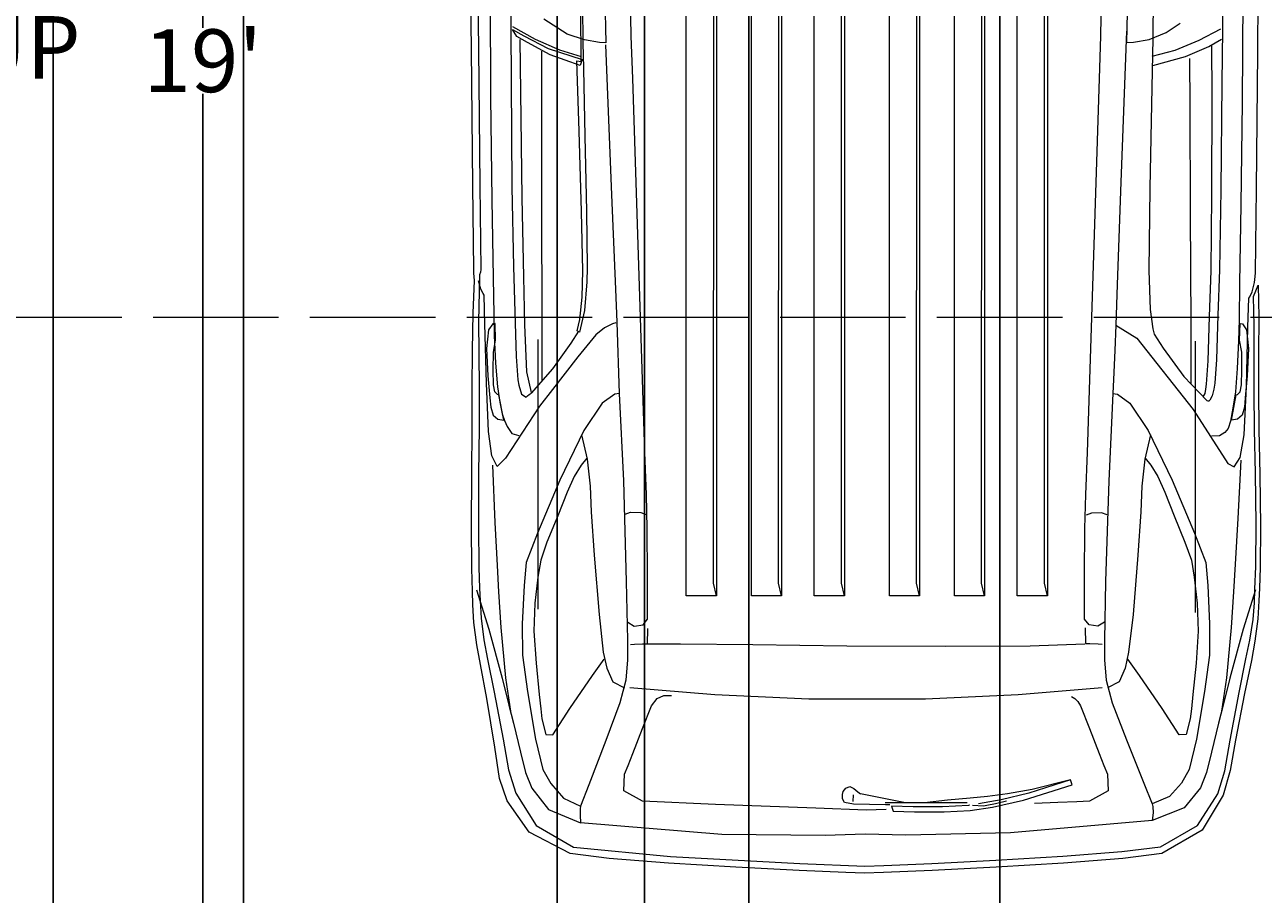
# Model space of a CAD drawing. Units: inches. Extents: x -36 to 401, y -686 to 73.
# Tile 4 of 15: x 184 to 303, y -615 to -532. Entities that reach past the tile are written whole.
import ezdxf

# ---------------------------------------------------------------- set-up
doc = ezdxf.new("R2010")
doc.units = ezdxf.units.IN
doc.header["$MEASUREMENT"] = 0
doc.linetypes.add('ACAD_ISO02W100', pattern=[15, 12, -3])
for name, color, linetype, lineweight in [('A-ANNO-DIMS', 2, 'Continuous', 18), ('A-ANNO-TEXT', 7, 'Continuous', 18), ('A-FLOR-OVHD', 8, 'ACAD_ISO02W100', 18), ('C-PKNG-VEHI', 8, 'Continuous', 13)]:
    doc.layers.add(name, color=color, linetype=linetype, lineweight=lineweight)
doc.styles.get("Standard").update_dxf_attribs({"font": 'arial.ttf'})
doc.dimstyles.get("Standard").update_dxf_attribs({"dimtxt": 0.18, "dimasz": 0.18, "dimexe": 0.18, "dimexo": 0.0625, "dimgap": 0.09, "dimtad": 0, "dimtih": 1, "dimtoh": 1, "dimdec": 0, "dimzin": 0, "dimdsep": 46, "dimlunit": 3, "dimtxsty": 'Standard', "dimcen": 0.09, "dimadec": 0, "dimazin": 0, "dimtfac": 1, "dimtdec": 0, "dimtofl": 0, "dimtmove": 0, "dimatfit": 3, "dimfxl": 1, "dimtolj": 1, "dimtzin": 0, "dimarcsym": 0})

# ---------------------------------------------------------------- blocks, each defined once
blk = doc.blocks.new('*D3')
at = {"layer": 'A-ANNO-DIMS', "color": 0, "lineweight": -2, "transparency": 16777216}
for p, q in [((200.9, -421.21), (201.62, -421.21)), ((201.44, -421.39), (201.44, -532.06)), ((201.44, -649.03), (201.44, -538.36)), ((200.9, -649.21), (201.62, -649.21))]:
    blk.add_line(p, q, dxfattribs=at)
at = {"layer": 'A-ANNO-DIMS', "color": 0, "transparency": 16777216}
for points in [[(201.41, -421.39), (201.47, -421.39), (201.44, -421.21)], [(201.41, -649.03), (201.47, -649.03), (201.44, -649.21)]]:
    blk.add_solid(points, dxfattribs=at)
at = {"layer": 'Defpoints', "color": 0, "transparency": 16777216}
for p in [(200.84, -421.21), (200.84, -649.21), (201.44, -649.21)]:
    blk.add_point(p, dxfattribs=at)
at = {"layer": 'A-ANNO-DIMS', "color": 0, "transparency": 16777216, "insert": (201.44, -535.21), "char_height": 6, "attachment_point": 5}
blk.add_mtext("\\A1;19'", dxfattribs=at)
blk = doc.blocks.new('*D73')
at = {"layer": 'A-ANNO-DIMS', "color": 0, "lineweight": -2, "transparency": 16777216}
for p, q in [((177.19, -421.27), (177.19, -685.69)), ((253.69, -421.27), (253.69, -685.69)), ((177.37, -685.51), (214.9, -685.51)), ((253.51, -685.51), (215.98, -685.51))]:
    blk.add_line(p, q, dxfattribs=at)
at = {"layer": 'A-ANNO-DIMS', "color": 0, "transparency": 16777216}
for points in [[(177.37, -685.48), (177.37, -685.54), (177.19, -685.51)], [(253.51, -685.48), (253.51, -685.54), (253.69, -685.51)]]:
    blk.add_solid(points, dxfattribs=at)
at = {"layer": 'Defpoints', "color": 0, "transparency": 16777216}
for p in [(177.19, -421.21), (253.69, -421.21), (253.69, -685.51)]:
    blk.add_point(p, dxfattribs=at)
at = {"layer": 'A-ANNO-DIMS', "color": 0, "transparency": 16777216, "insert": (215.44, -685.51), "char_height": 0.18, "attachment_point": 5}
blk.add_mtext('\\A1;6\'-4 1/2"', dxfattribs=at)
blk = doc.blocks.new('*D74')
at = {"layer": 'A-ANNO-DIMS', "color": 0, "lineweight": -2, "transparency": 16777216}
for p, q in [((277.69, -412.27), (277.69, -685.69)), ((313.69, -421.27), (313.69, -685.69)), ((277.87, -685.51), (295.36, -685.51)), ((313.51, -685.51), (296.02, -685.51))]:
    blk.add_line(p, q, dxfattribs=at)
at = {"layer": 'A-ANNO-DIMS', "color": 0, "transparency": 16777216}
for points in [[(277.87, -685.48), (277.87, -685.54), (277.69, -685.51)], [(313.51, -685.48), (313.51, -685.54), (313.69, -685.51)]]:
    blk.add_solid(points, dxfattribs=at)
at = {"layer": 'Defpoints', "color": 0, "transparency": 16777216}
for p in [(277.69, -412.21), (313.69, -421.21), (313.69, -685.51)]:
    blk.add_point(p, dxfattribs=at)
at = {"layer": 'A-ANNO-DIMS', "color": 0, "transparency": 16777216, "insert": (295.69, -685.51), "char_height": 0.18, "attachment_point": 5}
blk.add_mtext('\\A1;3\'-0"', dxfattribs=at)
blk = doc.blocks.new('*D87')
at = {"layer": 'A-ANNO-DIMS', "color": 0, "lineweight": -2, "transparency": 16777216}
for p, q in [((243.7, -154.81), (243.7, -685.69)), ((187.11, -163.6), (187.11, -685.69)), ((187.29, -685.51), (214.86, -685.51)), ((243.52, -685.51), (215.95, -685.51))]:
    blk.add_line(p, q, dxfattribs=at)
at = {"layer": 'A-ANNO-DIMS', "color": 0, "transparency": 16777216}
for points in [[(187.29, -685.48), (187.29, -685.54), (187.11, -685.51)], [(243.52, -685.48), (243.52, -685.54), (243.7, -685.51)]]:
    blk.add_solid(points, dxfattribs=at)
at = {"layer": 'Defpoints', "color": 0, "transparency": 16777216}
for p in [(243.7, -154.75), (187.11, -163.53), (243.7, -685.51)]:
    blk.add_point(p, dxfattribs=at)
at = {"layer": 'A-ANNO-DIMS', "color": 0, "transparency": 16777216, "insert": (215.4, -685.51), "char_height": 0.18, "attachment_point": 5}
blk.add_mtext('\\A1;4\'-8 1/2"', dxfattribs=at)
blk = doc.blocks.new('*D91')
at = {"layer": 'A-ANNO-DIMS', "color": 0, "lineweight": -2, "transparency": 16777216}
for p, q in [((205.32, -404.21), (205.32, -685.69)), ((235.34, -404.21), (235.34, -685.69)), ((205.5, -685.51), (220, -685.51)), ((235.16, -685.51), (220.66, -685.51))]:
    blk.add_line(p, q, dxfattribs=at)
at = {"layer": 'A-ANNO-DIMS', "color": 0, "transparency": 16777216}
for points in [[(205.5, -685.48), (205.5, -685.54), (205.32, -685.51)], [(235.16, -685.48), (235.16, -685.54), (235.34, -685.51)]]:
    blk.add_solid(points, dxfattribs=at)
at = {"layer": 'Defpoints', "color": 0, "transparency": 16777216}
for p in [(205.32, -404.14), (235.34, -404.14), (235.34, -685.51)]:
    blk.add_point(p, dxfattribs=at)
at = {"layer": 'A-ANNO-DIMS', "color": 0, "transparency": 16777216, "insert": (220.33, -685.51), "char_height": 0.18, "attachment_point": 5}
blk.add_mtext('\\A1;2\'-6"', dxfattribs=at)

msp = doc.modelspace()

# ---------------------------------------------------------------- linework, layer by layer
at = {"layer": 'A-FLOR-OVHD'}
msp.add_line((358.69, -559.77), (26.38, -559.77), dxfattribs=at)
at = {"layer": 'C-PKNG-VEHI'}
for p, q in [((247.7, -586.39), (247.7, -510.52)), ((250.3, -585.18), (250.33, -510.76)), ((250.59, -510.52), (250.59, -586.39)), ((250.59, -510.52), (250.59, -586.39)), ((253.93, -586.39), (253.93, -510.52)), ((256.53, -585.18), (256.56, -510.76)), ((256.82, -510.52), (256.82, -586.39)), ((256.82, -510.52), (256.82, -586.39)), ((259.94, -586.39), (259.94, -510.52)), ((262.54, -585.18), (262.57, -510.76)), ((262.83, -510.52), (262.83, -586.39)), ((262.83, -510.52), (262.83, -586.39)), ((267.13, -586.39), (267.13, -510.52)), ((269.73, -585.18), (269.76, -510.76)), ((270.02, -510.52), (270.02, -586.39)), ((270.02, -510.52), (270.02, -586.39)), ((273.36, -586.39), (273.36, -510.52)), ((275.96, -585.18), (275.98, -510.76)), ((276.24, -510.52), (276.24, -586.39)), ((276.25, -510.52), (276.25, -586.39)), ((279.36, -586.39), (279.36, -510.52)), ((281.97, -585.18), (281.99, -510.76)), ((282.25, -510.52), (282.25, -586.39)), ((230.89, -525.47), (230.92, -532.14)), ((239.84, -525.17), (240, -533.51)), ((290.03, -525.48), (289.82, -533.45)), ((292.4, -525.48), (292.33, -533.09)), ((298.98, -525.86), (299.01, -532.23)), ((227.14, -534.09), (227.08, -527.24)), ((227.75, -527.24), (227.81, -534.08)), ((228.92, -528.19), (228.98, -538.68)), ((302.39, -534.4), (302.45, -527.56)), ((242.43, -532.86), (242.36, -529.15)), ((287.38, -532.86), (287.43, -529.15)), ((300.95, -528.69), (300.9, -539.19)), ((237.63, -535.28), (237.61, -530.43)), ((237.77, -530.16), (237.8, -533.34)), ((231.07, -531.94), (233.23, -533.15)), ((236.31, -532.67), (234.07, -531.23)), ((293.63, -532.52), (294.95, -531.6)), ((230.92, -532.14), (230.94, -537.2)), ((231.47, -532.89), (231.08, -532.22)), ((231.08, -532.22), (232.14, -532.84)), ((232.5, -533.48), (231.47, -532.89)), ((231.78, -533.17), (231.83, -538.21)), ((232.14, -532.84), (234.49, -534.03)), ((233.23, -533.15), (235.56, -534.17)), ((237.96, -533.21), (236.31, -532.67)), ((239.39, -533.45), (237.96, -533.21)), ((242.58, -536.92), (242.43, -532.86)), ((287.23, -536.92), (287.38, -532.86)), ((289.82, -532.37), (289.28, -546.84)), ((290.49, -533.42), (292, -533.19)), ((292, -533.19), (293.63, -532.52)), ((292.33, -533.09), (292.24, -537.78)), ((296.74, -533.26), (294.45, -534.23)), ((298.81, -532.2), (296.74, -533.26)), ((297.69, -533.84), (298.93, -533.16)), ((299.01, -532.23), (298.96, -537.34)), ((227.26, -547.15), (227.14, -534.09)), ((227.81, -534.08), (227.93, -547.13)), ((234.68, -534.63), (232.5, -533.48)), ((233.84, -534.28), (233.86, -549.32)), ((234.49, -534.03), (237.74, -535.08)), ((235.56, -534.17), (237.65, -534.81)), ((237.8, -533.34), (237.81, -533.66)), ((237.81, -533.66), (237.82, -534.57)), ((240, -533.51), (239.39, -533.45)), ((239.98, -533.7), (240.55, -548.04)), ((289.82, -533.45), (290.49, -533.42)), ((294.45, -534.23), (292.26, -534.82)), ((295.47, -534.8), (297.69, -533.84)), ((297.97, -533.75), (297.98, -538.5)), ((302.27, -547.45), (302.39, -534.4)), ((237.55, -535.67), (234.68, -534.63)), ((237.44, -541.96), (237.23, -535.23)), ((237.23, -535.23), (237.63, -535.28)), ((237.74, -535.08), (237.55, -535.67)), ((237.82, -534.57), (237.85, -535.97)), ((292.33, -535.68), (295.47, -534.8)), ((295.85, -534.98), (295.87, -539.57)), ((237.85, -535.97), (237.99, -542.43)), ((230.94, -537.2), (231.02, -547.31)), ((242.84, -544.89), (242.58, -536.92)), ((286.97, -544.89), (287.23, -536.92)), ((292.24, -537.78), (292.06, -547.39)), ((298.96, -537.34), (298.86, -547.56)), ((228.98, -538.68), (229.1, -548.5)), ((231.83, -538.21), (231.96, -548.31)), ((297.98, -538.5), (297.97, -548.04)), ((300.9, -539.19), (300.77, -549)), ((295.87, -539.57), (295.92, -549.82)), ((237.68, -549.63), (237.44, -541.96)), ((237.99, -542.43), (238.15, -549.59)), ((243.16, -554.81), (242.84, -544.89)), ((286.66, -554.81), (286.97, -544.89)), ((227.37, -555.2), (227.26, -547.15)), ((227.93, -547.13), (228.03, -555.17)), ((231.02, -547.31), (231.15, -554.9)), ((289.28, -546.84), (288.94, -556.63)), ((292.06, -547.39), (291.97, -555.28)), ((302.16, -555.49), (302.27, -547.45)), ((229.1, -548.5), (229.22, -555.99)), ((231.96, -548.31), (232.11, -555.89)), ((240.55, -548.04), (240.92, -557.07)), ((297.97, -548.04), (297.88, -555.32)), ((298.86, -547.56), (298.72, -555.21)), ((233.86, -549.32), (233.87, -560.07)), ((237.81, -555.31), (237.68, -549.63)), ((238.15, -549.59), (238.23, -554.98)), ((295.92, -549.82), (295.97, -560.44)), ((300.77, -549), (300.65, -556.49)), ((227.38, -555.54), (227.37, -555.2)), ((227.39, -555.88), (227.38, -555.54)), ((227.92, -555.7), (227.91, -555.97)), ((228, -555.45), (227.92, -555.7)), ((228.03, -555.17), (228, -555.45)), ((231.15, -554.9), (231.29, -559.26)), ((237.73, -557.82), (237.81, -555.31)), ((238.23, -554.98), (238.18, -556.35)), ((243.47, -564.73), (243.16, -554.81)), ((286.34, -564.73), (286.66, -554.81)), ((291.97, -555.28), (292.1, -559)), ((297.88, -555.32), (297.74, -559.68)), ((298.72, -555.21), (298.57, -559.56)), ((302.14, -555.84), (302.16, -555.49)), ((227.32, -559.36), (227.44, -556.22)), ((227.44, -556.22), (227.39, -555.88)), ((228.04, -557.06), (227.82, -556.28)), ((227.91, -555.97), (227.89, -557.28)), ((229.22, -555.99), (229.28, -559.49)), ((232.11, -555.89), (232.22, -560.47)), ((238.18, -556.35), (237.97, -559.09)), ((288.94, -556.63), (288.81, -560.5)), ((300.65, -556.49), (300.59, -560)), ((301.85, -557.31), (302.07, -556.43)), ((301.97, -557.75), (302.43, -556.68)), ((302.07, -556.43), (302.11, -556.15)), ((302.11, -556.15), (302.14, -555.84)), ((302.43, -556.68), (302.5, -559.75)), ((227.89, -557.28), (227.82, -560.14)), ((228.25, -557.49), (228.04, -557.06)), ((228.35, -557.63), (228.25, -557.49)), ((228.41, -560.39), (228.35, -557.63)), ((237.5, -559.96), (237.73, -557.82)), ((240.92, -557.07), (241.06, -560.21)), ((301.45, -560.7), (301.52, -557.93)), ((301.52, -557.93), (301.62, -557.79)), ((301.62, -557.79), (301.85, -557.31)), ((302.05, -560.58), (301.97, -557.75)), ((227.24, -562.91), (227.32, -559.36)), ((231.29, -559.26), (231.43, -563.49)), ((237.97, -559.09), (237.48, -561.17)), ((292.1, -559), (292.34, -560.87)), ((227.82, -560.14), (227.85, -563.18)), ((228.57, -566.06), (228.41, -560.39)), ((229.18, -560.38), (228.77, -560.95)), ((229.4, -560.34), (229.18, -560.38)), ((229.28, -559.49), (229.33, -561.49)), ((229.44, -561.95), (229.4, -560.34)), ((232.22, -560.47), (232.4, -564.97)), ((233.87, -560.07), (233.88, -565.81)), ((237.26, -561.06), (237.5, -559.96)), ((240.63, -560.39), (239.87, -560.77)), ((240.97, -560.27), (240.63, -560.39)), ((241.06, -560.21), (241.28, -567.03)), ((288.81, -560.5), (288.7, -562.93)), ((288.81, -560.5), (290.82, -561.74)), ((295.97, -560.44), (295.99, -566.12)), ((297.74, -559.68), (297.6, -563.91)), ((298.57, -559.56), (298.43, -563.8)), ((300.59, -560), (300.55, -561.99)), ((300.65, -561.95), (300.69, -560.34)), ((300.69, -560.34), (300.92, -560.38)), ((300.92, -560.38), (301.32, -560.95)), ((302.5, -559.75), (302.47, -563.18)), ((228.77, -560.95), (228.59, -562.75)), ((229.33, -561.49), (229.45, -564.15)), ((237.39, -561.07), (236.65, -562.22)), ((237.48, -561.17), (237.26, -561.06)), ((239.05, -561.43), (237.33, -563.55)), ((239.87, -560.77), (239.05, -561.43)), ((290.82, -561.74), (296.21, -568.56)), ((292.34, -560.87), (292.47, -561.38)), ((292.47, -561.38), (293.33, -562.7)), ((301.3, -566.37), (301.45, -560.7)), ((301.32, -560.95), (301.5, -562.75)), ((302.04, -563.54), (302.05, -560.58)), ((227.22, -566.52), (227.24, -562.91)), ((228.59, -562.75), (228.72, -565.34)), ((229.24, -563.08), (229.44, -561.95)), ((233.5, -561.87), (233.5, -587.68)), ((236.65, -562.22), (234.9, -564.69)), ((293.33, -562.7), (295.3, -565.42)), ((296.41, -562.05), (296.41, -588)), ((300.55, -561.99), (300.42, -564.65)), ((300.86, -563.08), (300.65, -561.95)), ((301.5, -562.75), (301.37, -565.34)), ((227.85, -563.18), (227.89, -566.52)), ((229.23, -564.82), (229.24, -563.08)), ((231.43, -563.49), (231.58, -565.74)), ((237.33, -563.55), (234.9, -566.66)), ((288.7, -562.93), (288.58, -565.7)), ((297.6, -563.91), (297.45, -566.16)), ((298.43, -563.8), (298.29, -566.05)), ((300.86, -564.82), (300.86, -563.08)), ((302.03, -566.85), (302.04, -563.54)), ((302.47, -563.18), (302.44, -566.74)), ((229.26, -566.21), (229.23, -564.82)), ((229.45, -564.15), (229.64, -566.39)), ((232.4, -564.97), (232.84, -566.96)), ((234.9, -564.69), (232.84, -567.01)), ((243.73, -572.68), (243.47, -564.73)), ((286.08, -572.68), (286.34, -564.73)), ((300.42, -564.65), (300.24, -566.89)), ((300.83, -566.21), (300.86, -564.82)), ((228.78, -570.69), (228.57, -566.06)), ((228.72, -565.34), (228.9, -567.46)), ((229.39, -566.87), (229.26, -566.21)), ((229.64, -566.39), (229.86, -567.88)), ((231.58, -565.74), (231.67, -566.25)), ((231.67, -566.25), (231.94, -567.12)), ((288.58, -565.7), (288.52, -567.03)), ((295.3, -565.42), (297.5, -567.7)), ((297.45, -566.16), (297.38, -566.63)), ((298.29, -566.05), (298.17, -566.63)), ((300.7, -566.87), (300.83, -566.21)), ((301.09, -571), (301.3, -566.37)), ((301.37, -565.34), (301.19, -567.46)), ((227.2, -570.33), (227.22, -566.52)), ((227.89, -566.52), (227.87, -570.33)), ((228.9, -567.46), (228.99, -568.34)), ((229.63, -567.13), (229.39, -566.87)), ((229.76, -567.18), (229.63, -567.13)), ((230.23, -569.6), (229.76, -567.18)), ((231.94, -567.12), (232.37, -567.39)), ((232.37, -567.39), (232.52, -567.28)), ((232.52, -567.28), (232.68, -567.15)), ((232.68, -567.15), (232.84, -567.01)), ((234.9, -566.66), (233.66, -568.25)), ((240.85, -567.11), (239.66, -567.98)), ((241.28, -567.03), (240.85, -567.11)), ((241.28, -567.03), (241.68, -575.4)), ((288.52, -567.03), (288.12, -575.4)), ((288.52, -567.03), (288.95, -567.11)), ((288.95, -567.11), (290.13, -567.98)), ((297.31, -567.03), (297.13, -567.35)), ((297.38, -566.63), (297.31, -567.03)), ((298.02, -567.25), (297.81, -567.69)), ((298.17, -566.63), (298.02, -567.25)), ((299.86, -569.6), (300.33, -567.18)), ((300.24, -566.89), (300.01, -568.45)), ((300.33, -567.18), (300.46, -567.13)), ((300.46, -567.13), (300.7, -566.87)), ((301.19, -567.46), (301.1, -568.34)), ((302.08, -570.52), (302.03, -566.85)), ((302.44, -566.74), (302.5, -570.49)), ((228.99, -568.34), (229.21, -569.12)), ((229.86, -567.88), (230.07, -568.99)), ((233.66, -568.25), (230.39, -573.24)), ((239.66, -567.98), (237.88, -570.57)), ((290.13, -567.98), (291.91, -570.57)), ((296.21, -568.56), (299.52, -573.74)), ((297.5, -567.7), (297.61, -567.75)), ((297.61, -567.75), (297.72, -567.75)), ((297.72, -567.75), (297.81, -567.69)), ((300.01, -568.45), (299.78, -569.68)), ((301.1, -568.34), (300.88, -569.12)), ((229.21, -569.12), (229.65, -569.49)), ((229.65, -569.49), (230.23, -569.6)), ((230.07, -568.99), (230.29, -569.62)), ((230.29, -569.62), (230.55, -570.21)), ((299.78, -569.68), (299.55, -570.38)), ((300.45, -569.49), (299.86, -569.6)), ((300.88, -569.12), (300.45, -569.49)), ((227.17, -574.72), (227.2, -570.33)), ((227.87, -570.33), (227.83, -574.72)), ((229.09, -573.01), (228.78, -570.69)), ((230.55, -570.21), (230.99, -570.88)), ((230.99, -570.88), (231.67, -571.05)), ((237.88, -570.57), (235.61, -575.34)), ((237.67, -571), (238.21, -573.31)), ((292.13, -571), (291.58, -573.31)), ((291.91, -570.57), (294.19, -575.34)), ((298.73, -571.08), (297.97, -571.13)), ((299.24, -570.76), (298.73, -571.08)), ((299.55, -570.38), (299.24, -570.76)), ((300.7, -573.16), (301.09, -571)), ((302.17, -574.65), (302.08, -570.52)), ((302.5, -570.49), (302.59, -574.78)), ((229.61, -574.03), (229.09, -573.01)), ((230.39, -573.24), (229.61, -574.03)), ((238.17, -573.24), (237.64, -573.89)), ((238.21, -573.31), (238.49, -575.91)), ((243.88, -576.71), (243.73, -572.68)), ((285.94, -576.71), (286.08, -572.68)), ((291.58, -573.31), (291.3, -575.91)), ((291.62, -573.24), (292.16, -573.89)), ((300.12, -574.06), (300.7, -573.16)), ((300.75, -573.41), (300.49, -579.01)), ((227.15, -579.74), (227.17, -574.72)), ((227.83, -574.72), (227.82, -579.74)), ((229.16, -573.91), (229.39, -579.38)), ((237.64, -573.89), (236.97, -574.97)), ((292.16, -573.89), (292.82, -574.97)), ((299.52, -573.74), (300.12, -574.06)), ((302.22, -579.53), (302.17, -574.65)), ((235.61, -575.34), (233.46, -580.41)), ((236.97, -574.97), (236.29, -576.49)), ((238.49, -575.91), (238.6, -578.37)), ((241.68, -575.4), (241.96, -585.02)), ((288.12, -575.4), (287.83, -585.02)), ((291.3, -575.91), (291.19, -578.37)), ((292.82, -574.97), (293.5, -576.49)), ((294.19, -575.34), (296.33, -580.41)), ((302.59, -574.78), (302.65, -579.74)), ((236.29, -576.49), (235.4, -578.74)), ((243.96, -579.95), (243.88, -576.71)), ((285.85, -579.95), (285.94, -576.71)), ((293.5, -576.49), (294.4, -578.74)), ((229.39, -579.38), (229.59, -583.49)), ((235.4, -578.74), (234.37, -581.27)), ((238.6, -578.37), (238.87, -582.52)), ((241.85, -578.58), (242.37, -578.41)), ((242.37, -578.41), (243.35, -578.42)), ((243.35, -578.42), (243.86, -578.62)), ((286.47, -578.48), (285.95, -578.68)), ((287.44, -578.47), (286.47, -578.48)), ((287.97, -578.64), (287.44, -578.47)), ((291.19, -578.37), (290.92, -582.52)), ((294.4, -578.74), (295.42, -581.27)), ((300.49, -579.01), (300.23, -583.36)), ((227.18, -583.79), (227.15, -579.74)), ((227.82, -579.74), (227.85, -583.7)), ((233.46, -580.41), (232.39, -583.21)), ((244, -584.47), (243.96, -579.95)), ((285.82, -584.47), (285.85, -579.95)), ((296.33, -580.41), (297.4, -583.21)), ((302.19, -583.59), (302.22, -579.53)), ((302.65, -579.74), (302.61, -583.7)), ((234.37, -581.27), (233.77, -582.99)), ((295.42, -581.27), (296.03, -582.99)), ((233.77, -582.99), (233.48, -584.61)), ((238.87, -582.52), (239.35, -588.17)), ((290.92, -582.52), (290.45, -588.17)), ((296.03, -582.99), (296.31, -584.61)), ((227.24, -585.95), (227.18, -583.79)), ((227.85, -583.7), (227.92, -585.68)), ((229.59, -583.49), (229.72, -586.02)), ((232.39, -583.21), (232.17, -585.41)), ((297.4, -583.21), (297.62, -585.41)), ((300.23, -583.36), (300.07, -586.02)), ((302.12, -585.75), (302.19, -583.59)), ((302.61, -583.7), (302.54, -585.68)), ((232.17, -585.41), (232.01, -589.07)), ((233.48, -584.61), (233.2, -587.1)), ((241.96, -585.02), (242.07, -590.65)), ((244, -588.64), (244, -584.47)), ((250.59, -586.39), (250.3, -585.18)), ((256.82, -586.39), (256.53, -585.18)), ((262.83, -586.39), (262.54, -585.18)), ((270.02, -586.39), (269.73, -585.18)), ((276.24, -586.39), (275.96, -585.18)), ((282.25, -586.39), (281.97, -585.18)), ((285.82, -588.64), (285.82, -584.47)), ((287.83, -585.02), (287.72, -590.65)), ((296.31, -584.61), (296.59, -587.1)), ((297.62, -585.41), (297.78, -589.07)), ((227.27, -587.26), (227.24, -585.95)), ((227.63, -585.81), (228.82, -589.6)), ((227.92, -585.68), (227.96, -586.89)), ((229.72, -586.02), (229.96, -589.42)), ((250.59, -586.39), (247.7, -586.39)), ((256.82, -586.39), (253.93, -586.39)), ((262.83, -586.39), (259.94, -586.39)), ((270.02, -586.39), (267.13, -586.39)), ((276.25, -586.39), (273.36, -586.39)), ((282.25, -586.39), (279.36, -586.39)), ((300.07, -586.02), (299.84, -589.42)), ((302.17, -585.81), (300.98, -589.6)), ((302.08, -587.07), (302.12, -585.75)), ((302.54, -585.68), (302.5, -586.89)), ((227.38, -588.96), (227.27, -587.26)), ((227.96, -586.89), (228.07, -588.53)), ((233.2, -587.1), (233.12, -589.78)), ((296.59, -587.1), (296.68, -589.78)), ((301.95, -588.66), (302.08, -587.07)), ((302.5, -586.89), (302.39, -588.59)), ((227.65, -591.09), (227.38, -588.96)), ((228.07, -588.53), (228.33, -590.61)), ((239.35, -588.17), (239.76, -591.8)), ((242.1, -588.92), (242.72, -589.3)), ((243.57, -589.18), (244, -588.64)), ((286.24, -589.18), (285.82, -588.64)), ((287.71, -588.92), (287.09, -589.3)), ((290.45, -588.17), (290.03, -591.8)), ((301.62, -590.64), (301.95, -588.66)), ((302.39, -588.59), (302.12, -590.72)), ((228.82, -589.6), (230.07, -594.27)), ((229.96, -589.42), (230.4, -594.24)), ((232.01, -589.07), (232.03, -592.09)), ((233.12, -589.78), (233.32, -592.83)), ((242.72, -589.3), (243.57, -589.18)), ((244, -589.53), (243.95, -591.01)), ((285.86, -589.46), (285.91, -590.95)), ((287.09, -589.3), (286.24, -589.18)), ((296.68, -589.78), (296.48, -592.83)), ((297.78, -589.07), (297.76, -592.09)), ((299.84, -589.42), (299.39, -594.24)), ((300.98, -589.6), (299.72, -594.27)), ((228, -592.97), (227.65, -591.09)), ((228.33, -590.61), (228.67, -592.45)), ((242.07, -590.65), (242.08, -592.52)), ((242.74, -591.06), (242.36, -591.08)), ((243.52, -591.03), (242.74, -591.06)), ((243.95, -591.01), (243.52, -591.03)), ((247.16, -591.02), (243.95, -591.01)), ((254.08, -591.1), (247.16, -591.02)), ((263.07, -591.2), (254.08, -591.1)), ((272.46, -591.25), (263.07, -591.2)), ((280.61, -591.2), (272.46, -591.25)), ((285.84, -591.01), (280.61, -591.2)), ((285.91, -590.95), (286.33, -590.97)), ((286.33, -590.97), (287.12, -591)), ((287.12, -591), (287.5, -591.02)), ((287.72, -590.65), (287.72, -592.52)), ((301.25, -592.43), (301.62, -590.64)), ((302.12, -590.72), (301.77, -592.6)), ((228.67, -592.45), (229.33, -595.61)), ((232.03, -592.09), (232.49, -595.56)), ((238.74, -594.02), (239.83, -592.45)), ((239.76, -591.8), (240.09, -593.31)), ((242.08, -592.52), (241.92, -594.48)), ((287.72, -592.52), (287.87, -594.48)), ((290.03, -591.8), (289.7, -593.31)), ((291.06, -594.02), (289.96, -592.45)), ((297.76, -592.09), (297.3, -595.56)), ((300.59, -595.63), (301.25, -592.43)), ((228.61, -596.21), (228, -592.97)), ((233.32, -592.83), (233.61, -595.85)), ((240.09, -593.31), (240.68, -594.61)), ((289.7, -593.31), (289.11, -594.61)), ((296.48, -592.83), (296.18, -595.85)), ((301.77, -592.6), (301.12, -595.74)), ((230.07, -594.27), (230.73, -596.86)), ((230.4, -594.24), (230.88, -597.44)), ((236.55, -597.19), (238.74, -594.02)), ((240.68, -594.61), (241.78, -595.2)), ((241.92, -594.48), (241.35, -596.64)), ((287.87, -594.48), (288.44, -596.64)), ((289.11, -594.61), (288.01, -595.2)), ((293.25, -597.19), (291.06, -594.02)), ((299.39, -594.24), (298.92, -597.44)), ((299.72, -594.27), (299.06, -596.86)), ((229.33, -595.61), (230.19, -600.11)), ((232.49, -595.56), (233.28, -600.11)), ((233.61, -595.85), (233.77, -597.22)), ((250.42, -595.88), (242.29, -595.2)), ((244.9, -596.21), (245.56, -595.92)), ((245.56, -595.92), (246.29, -595.92)), ((259.42, -596.27), (250.42, -595.88)), ((279.45, -595.88), (270.59, -596.27)), ((287.5, -595.2), (279.45, -595.88)), ((284.57, -596.02), (284.89, -596.21)), ((296.18, -595.85), (296.03, -597.22)), ((297.3, -595.56), (296.51, -600.11)), ((299.73, -600.19), (300.59, -595.63)), ((301.12, -595.74), (300.26, -600.21)), ((229.38, -600.86), (228.61, -596.21)), ((230.73, -596.86), (231.16, -598.59)), ((233.77, -597.22), (233.89, -598.16)), ((234.92, -599.68), (236.55, -597.19)), ((241.35, -596.64), (239.99, -600.23)), ((243.51, -599.08), (244.38, -596.93)), ((244.38, -596.93), (244.9, -596.21)), ((265.04, -596.28), (259.42, -596.27)), ((270.59, -596.27), (265.04, -596.28)), ((284.89, -596.21), (285.17, -596.5)), ((285.17, -596.5), (285.41, -596.93)), ((285.41, -596.93), (286.28, -599.08)), ((288.44, -596.64), (289.83, -600.17)), ((294.87, -599.68), (293.25, -597.19)), ((296.03, -597.22), (295.91, -598.16)), ((299.06, -596.86), (298.63, -598.59)), ((233.89, -598.16), (234.27, -599.65)), ((295.91, -598.16), (295.53, -599.65)), ((231.16, -598.59), (231.84, -601.36)), ((234.27, -599.65), (234.92, -599.68)), ((242.58, -601.49), (243.51, -599.08)), ((286.28, -599.08), (287.21, -601.49)), ((295.53, -599.65), (294.87, -599.68)), ((298.63, -598.59), (297.95, -601.36)), ((230.19, -600.11), (230.7, -603.03)), ((233.28, -600.11), (233.98, -603)), ((239.99, -600.23), (238.37, -604.48)), ((289.83, -600.17), (291.49, -604.31)), ((296.51, -600.11), (295.81, -603)), ((299.22, -603.14), (299.73, -600.19)), ((300.26, -600.21), (299.75, -603.11)), ((229.84, -603.86), (229.38, -600.86)), ((231.84, -601.36), (232.32, -603.29)), ((242.14, -602.64), (242.58, -601.49)), ((287.21, -601.49), (287.65, -602.64)), ((297.95, -601.36), (297.47, -603.29)), ((230.7, -603.03), (231.38, -605.26)), ((233.98, -603), (234.73, -604.36)), ((241.78, -603.47), (242.14, -602.64)), ((287.65, -602.64), (288.02, -603.47)), ((295.81, -603), (295.09, -604.31)), ((298.55, -605.33), (299.22, -603.14)), ((299.75, -603.11), (299.09, -605.47)), ((230.56, -606.02), (229.84, -603.86)), ((232.32, -603.29), (232.91, -604.81)), ((234.73, -604.36), (235.94, -605.74)), ((241.72, -605.06), (241.78, -603.47)), ((284.47, -604), (280.49, -605.29)), ((284.47, -604), (280.81, -604.92)), ((284.62, -604.48), (284.47, -604)), ((288.02, -603.47), (288.08, -605.06)), ((291.49, -604.31), (292.29, -606.31)), ((295.09, -604.31), (293.93, -605.58)), ((297.47, -603.29), (296.91, -604.75)), ((231.38, -605.26), (233.34, -608.37)), ((232.91, -604.81), (234.53, -606.83)), ((238.37, -604.48), (237.59, -606.53)), ((243.52, -606.03), (241.72, -605.06)), ((262.65, -605.39), (262.72, -605.11)), ((262.66, -605.81), (262.65, -605.39)), ((262.72, -605.11), (262.98, -604.79)), ((262.98, -604.79), (263.34, -604.64)), ((263.34, -604.64), (263.74, -604.82)), ((263.66, -606.08), (263.71, -605.43)), ((263.74, -604.82), (264.1, -605.15)), ((264.1, -605.15), (264.36, -605.35)), ((264.68, -605.4), (264.36, -605.35)), ((265.96, -605.65), (264.68, -605.4)), ((276.51, -605.59), (274.88, -605.74)), ((278.43, -605.35), (276.51, -605.59)), ((280.49, -605.29), (277.84, -605.92)), ((280.81, -604.92), (278.43, -605.35)), ((279.98, -605.96), (284.62, -604.48)), ((288.08, -605.06), (286.28, -606.03)), ((293.93, -605.58), (292.29, -606.31)), ((296.91, -604.75), (295.33, -606.67)), ((296.61, -608.38), (298.55, -605.33)), ((299.09, -605.47), (297.06, -608.81)), ((232.68, -609.01), (230.56, -606.02)), ((235.94, -605.74), (237.59, -606.53)), ((237.59, -606.53), (237.56, -606.78)), ((250.5, -606.35), (243.52, -606.03)), ((260.08, -606.72), (250.5, -606.35)), ((264.9, -606.9), (260.08, -606.72)), ((262.85, -606.18), (262.66, -605.81)), ((263.71, -606.32), (262.85, -606.18)), ((266.75, -606.39), (263.71, -606.32)), ((268.68, -606.2), (265.96, -605.65)), ((268.98, -606.2), (266.72, -606.19)), ((267.17, -606.39), (266.75, -606.39)), ((269.4, -606.58), (267.35, -606.51)), ((267.35, -606.51), (267.5, -606.99)), ((272.65, -606.21), (268.98, -606.2)), ((272.22, -606.58), (269.4, -606.58)), ((272.7, -605.94), (270.5, -606.2)), ((274.72, -606.44), (272.22, -606.58)), ((274.57, -606.21), (272.65, -606.21)), ((274.88, -605.74), (272.7, -605.94)), ((274.75, -606.44), (274.72, -606.44)), ((274.77, -606.43), (274.75, -606.44)), ((274.8, -606.43), (274.77, -606.43)), ((274.86, -606.92), (277, -606.63)), ((276.14, -606.53), (275.09, -606.45)), ((277.84, -605.92), (275.65, -606.3)), ((276.47, -606.47), (276.14, -606.53)), ((277.29, -606.3), (276.47, -606.47)), ((277, -606.63), (279.98, -605.96)), ((278.35, -606.05), (277.29, -606.3)), ((283.26, -606.18), (281.02, -606.28)), ((285.06, -606.1), (283.26, -606.18)), ((286.28, -606.03), (285.06, -606.1)), ((292.29, -606.31), (292.33, -606.56)), ((295.33, -606.67), (292.29, -607.9)), ((292.33, -606.56), (292.36, -607.16)), ((234.53, -606.83), (237.59, -608.12)), ((237.56, -606.78), (237.53, -607.38)), ((237.53, -607.38), (237.59, -608.12)), ((266.82, -606.83), (264.9, -606.9)), ((267.5, -606.99), (269.55, -607.06)), ((269.55, -607.06), (272.37, -607.06)), ((272.37, -607.06), (274.86, -606.92)), ((292.29, -607.9), (278.72, -609.07)), ((292.36, -607.16), (292.29, -607.9)), ((236.59, -611.05), (232.68, -609.01)), ((233.34, -608.37), (236.9, -610.43)), ((251.11, -609.24), (237.59, -608.12)), ((278.72, -609.07), (268.72, -609.29)), ((293.07, -610.4), (296.61, -608.38)), ((297.06, -608.81), (293.2, -611.05)), ((260.99, -609.34), (251.11, -609.24)), ((264.82, -609.21), (260.99, -609.34)), ((268.72, -609.29), (264.82, -609.21)), ((240.31, -611.52), (236.59, -611.05)), ((236.9, -610.43), (246.19, -611.32)), ((246.19, -611.32), (258.57, -612)), ((277.31, -611.68), (283.73, -611.3)), ((283.73, -611.3), (289.37, -610.86)), ((289.37, -610.86), (293.07, -610.4)), ((293.2, -611.05), (289.48, -611.52)), ((245.99, -611.96), (240.31, -611.52)), ((252.45, -612.35), (245.99, -611.96)), ((258.5, -612.66), (252.45, -612.35)), ((262.98, -612.86), (258.5, -612.66)), ((258.57, -612), (264.77, -612.27)), ((264.77, -612.27), (266.59, -612.2)), ((271.22, -612.66), (266.58, -612.86)), ((266.59, -612.2), (271.2, -611.99)), ((271.2, -611.99), (277.31, -611.68)), ((277.35, -612.35), (271.22, -612.66)), ((283.81, -611.96), (277.35, -612.35)), ((289.48, -611.52), (283.81, -611.96)), ((264.74, -612.94), (262.98, -612.86)), ((266.58, -612.86), (264.74, -612.94))]:
    msp.add_line(p, q, dxfattribs=at)

# ---------------------------------------------------------------- texts
at = {"layer": 'A-ANNO-TEXT', "insert": (178.66, -530.94), "char_height": 6, "attachment_point": 1}
msp.add_mtext_dynamic_manual_height_columns('UP', width=0.1631, gutter_width=1, heights=[0], dxfattribs=at)

# ---------------------------------------------------------------- dimensions: what is measured, and where the dimension line sits
at = {"layer": 'A-ANNO-DIMS'}
for base, p1, p2, picture, middle in [((243.7, -685.51), (187.11, -163.53), (243.7, -154.75), '*D87', (215.4, -685.51)), ((235.34, -685.51), (205.32, -404.14), (235.34, -404.14), '*D91', (220.33, -685.51)), ((313.69, -685.51), (277.69, -412.21), (313.69, -421.21), '*D74', (295.69, -685.51)), ((253.69, -685.51), (177.19, -421.21), (253.69, -421.21), '*D73', (215.44, -685.51))]:
    dim = msp.add_linear_dim(base=base, p1=p1, p2=p2, dimstyle='Standard', override={"dimdec": 1, "dimlfac": 1, "dimrnd": 0, "dimzin": 1, "dimdsep": 46, "dimlunit": 4, "dimfrac": 2}, dxfattribs=at)
    dim.commit()
    dim.dimension.update_dxf_attribs({"geometry": picture, "text_midpoint": middle})
dim = msp.add_linear_dim(base=(201.44, -649.21), p1=(200.84, -421.21), p2=(200.84, -649.21), angle=90, dimstyle='Standard', override={"dimtxt": 6, "dimclrd": 0, "dimclre": 0, "dimclrt": 0}, dxfattribs=at)
dim.commit()
dim.dimension.update_dxf_attribs({"geometry": '*D3', "text_midpoint": (201.44, -535.21)})

doc.saveas('drawing.dxf')
